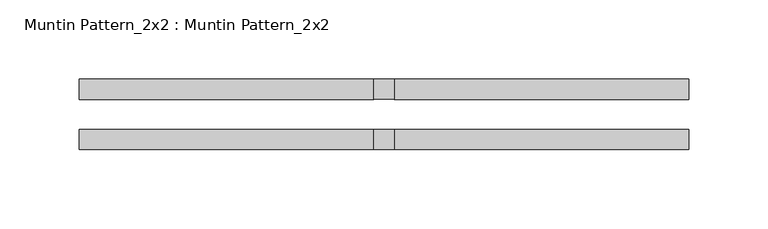
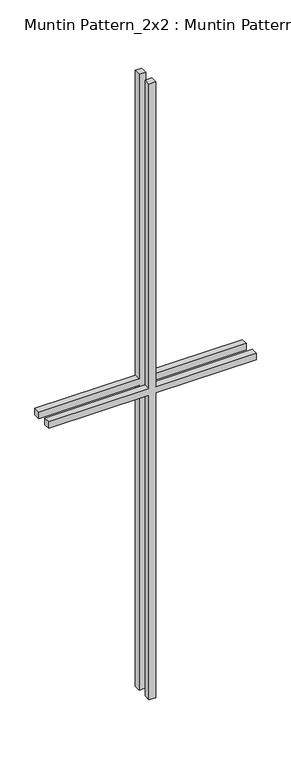
"""IFC4 building model written with IfcOpenShell, lengths in millimetres: proxy geometry, Muntin Pattern_2x2 : Muntin Pattern_2x2."""

from ifc_helpers import new_model, si_unit, frame, origin, place, context, project, spatial, polyline, outline, extrude, source, transform, mapped, element, save


def muntin_pattern_2x2_muntin_pattern_2x2_88bf7f41(model_context):
    return source(origin(), model_context, "Body", "SweptSolid", [
        extrude(outline(polyline([(609.6, -6.35), (609.6, -192.0875), (596.9, -192.0875), (596.9, -6.35), (0.0, -6.35), (0.0, 6.35), (596.9, 6.35), (596.9, 192.0875), (609.6, 192.0875), (609.6, 6.35), (1206.5, 6.35), (1206.5, -6.35), (609.6, -6.35)])), frame((0.0, 9.525, 0.0), z_axis=(0.0, 1.0, 0.0), x_axis=(0.0, 0.0, 1.0)), (0.0, 0.0, 1.0), 12.7),
        extrude(outline(polyline([(609.6, -6.35), (609.6, -192.0875), (596.9, -192.0875), (596.9, -6.35), (0.0, -6.35), (0.0, 6.35), (596.9, 6.35), (596.9, 192.0875), (609.6, 192.0875), (609.6, 6.35), (1206.5, 6.35), (1206.5, -6.35), (609.6, -6.35)])), frame((0.0, -22.225, 0.0), z_axis=(0.0, 1.0, 0.0), x_axis=(0.0, 0.0, 1.0)), (0.0, 0.0, 1.0), 12.7),
    ])


if __name__ == "__main__":
    model = new_model("IFC4")
    model_context = context("Model", 3, world=origin())
    ifc_project = project(units=[si_unit("LENGTHUNIT", "METRE", prefix="MILLI")], contexts=[model_context])
    site = spatial("IfcSite", under=ifc_project)
    building = spatial("IfcBuilding", under=site)
    placement = place(None, origin())
    muntin_pattern_2x2_muntin_pattern_2x2_shape = muntin_pattern_2x2_muntin_pattern_2x2_88bf7f41(model_context)
    element("IfcBuildingElementProxy", 1, Name="Muntin Pattern_2x2 : Muntin Pattern_2x2", ObjectType="Muntin Pattern_2x2 : Muntin Pattern_2x2", at=placement, inside=building, context=model_context, shape_type="MappedRepresentation", body=[
        mapped(muntin_pattern_2x2_muntin_pattern_2x2_shape, transform((0.0, 0.0, 0.0), x_axis=(1.0, 0.0, 0.0), y_axis=(0.0, 1.0, 0.0), z_axis=(0.0, 0.0, 1.0))),
    ])
    save(model, "model.ifc")

# Revit data of these elements
# Type "Muntin Pattern_2x2 : Muntin Pattern_2x2"
#   Width [instance default] = 4' - 0"
#   Thickness = 0' - 0 1/2"
#   Height [instance default] = 4' - 0"
#   Distance = 0' - 0 3/4"
#   Interior Material [instance default] = none
#   Exterior Material [instance default] = none
#   Default Elevation = 0
# Element 1 (IfcBuildingElementProxy, "Muntin Pattern_2x2 : Muntin Pattern_2x2")
#   Width = 1' - 3 1/8"
#   Height = 3' - 11 1/2"
#   Interior Material = Wood - Stained
#   Materials on its faces: "Wood - Stained"
# Materials
#   "Wood - Stained": class "Wood", colour RGB 224 178 126, transparency 0, Cost = 0
